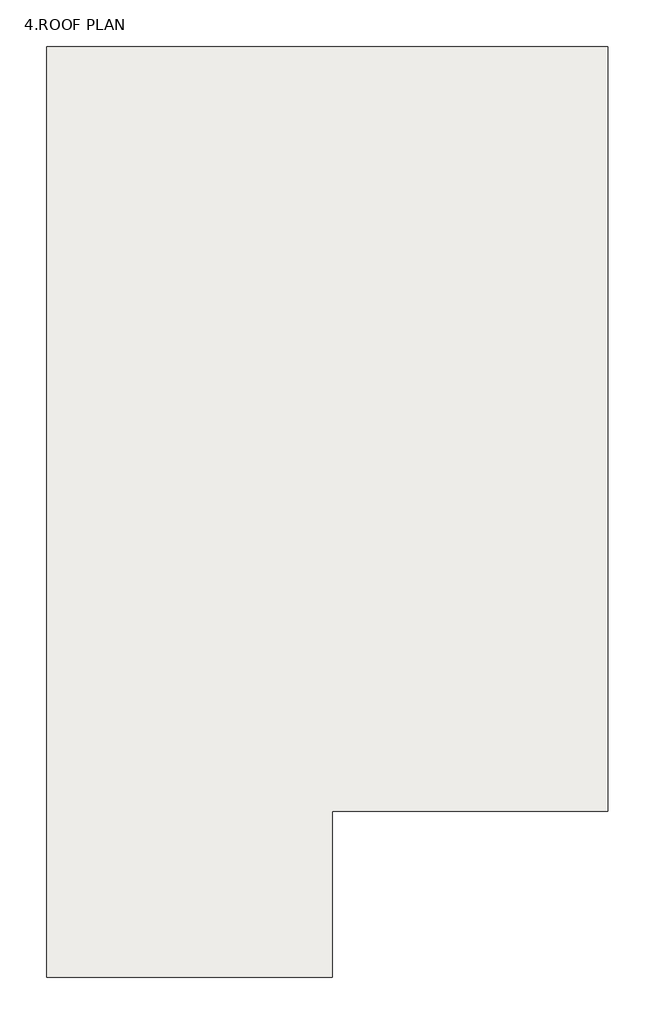
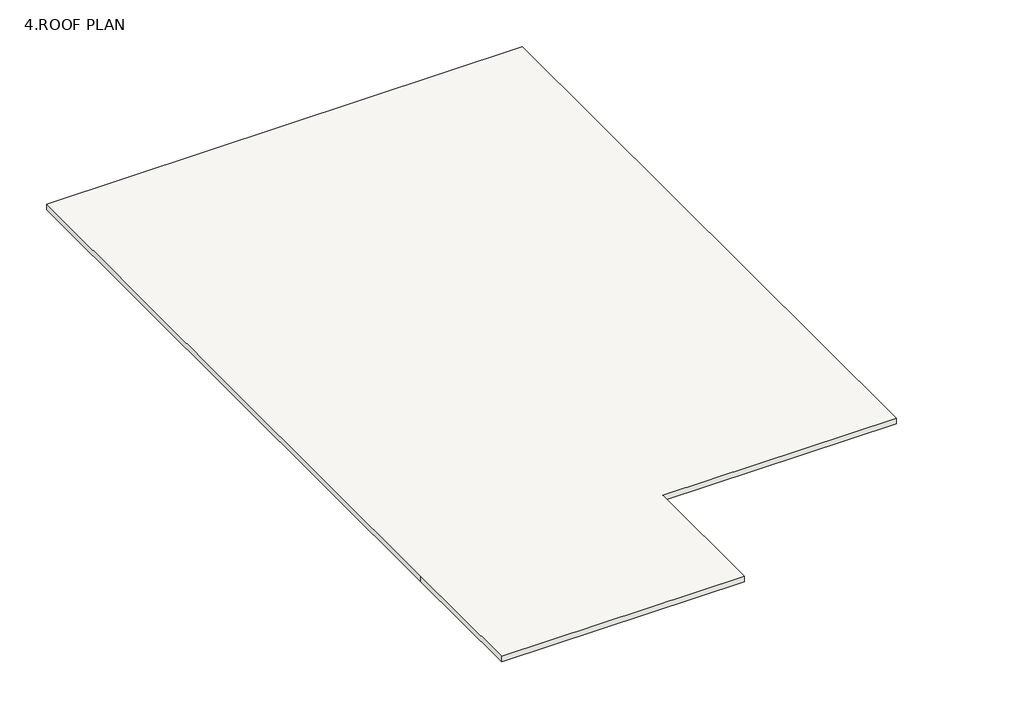
# One storey: 1 slab.
"""IFC4 building model written with IfcOpenShell, lengths in millimetres."""

from ifc_helpers import new_model, si_unit, frame, origin, place, context, project, spatial, polyline, outline, extrude, element, save

model = new_model("IFC4")

# Units and contexts
model_context = context("Model", 3, world=origin())
ifc_project = project(units=[si_unit("LENGTHUNIT", "METRE", prefix="MILLI")], contexts=[model_context])

# Site, building, storey
site = spatial("IfcSite", under=ifc_project)
building = spatial("IfcBuilding", under=site)
storey = spatial("IfcBuildingStorey", under=building, Name="4.ROOF PLAN", Elevation=6950.0)

# Slab
placement = place(None, origin())
element("IfcSlab", 1, ObjectType="6\" floor", at=placement, inside=storey, context=model_context, shape_type="SweptSolid", body=[
    extrude(outline(polyline([(-6341.6536251, 10590.826913), (5897.7463749, 10590.826913), (5897.7463749, -6077.173087), (-109.4536251, -6077.173087), (-109.4536251, -9703.573087), (-6341.6536251, -9703.573087), (-6341.6536251, -6077.173087), (-6341.6536251, 10590.826913)])), frame((0.0, 0.0, 7547.6), z_axis=(0.0, 0.0, 1.0), x_axis=(1.0, 0.0, 0.0)), (0.0, 0.0, 1.0), 152.4),
])

save(model, "model.ifc")

# Revit data of these elements
# Type "6\" floor"
#   Assembly Code = "B1010"
#   Function = 0
#   Layers, outside or top first: 0' - 6" "Laminate, Ivory, Matte" (function 1)
# Element 1 (IfcSlab, "6\" floor")
#   built-in parameter 1001955 = 3.14159 (stored number, unit not read)
#   Height Offset From Level = 2' - 5.52756"
#   Phase Created = New Construction
#   Materials on its faces: "Laminate, Ivory, Matte"
# Materials
#   "Laminate, Ivory, Matte": class "Plastic", colour RGB 247 247 239, transparency 0, Description = "Plastic Laminate - Ivory, Matte", Cost = 0
